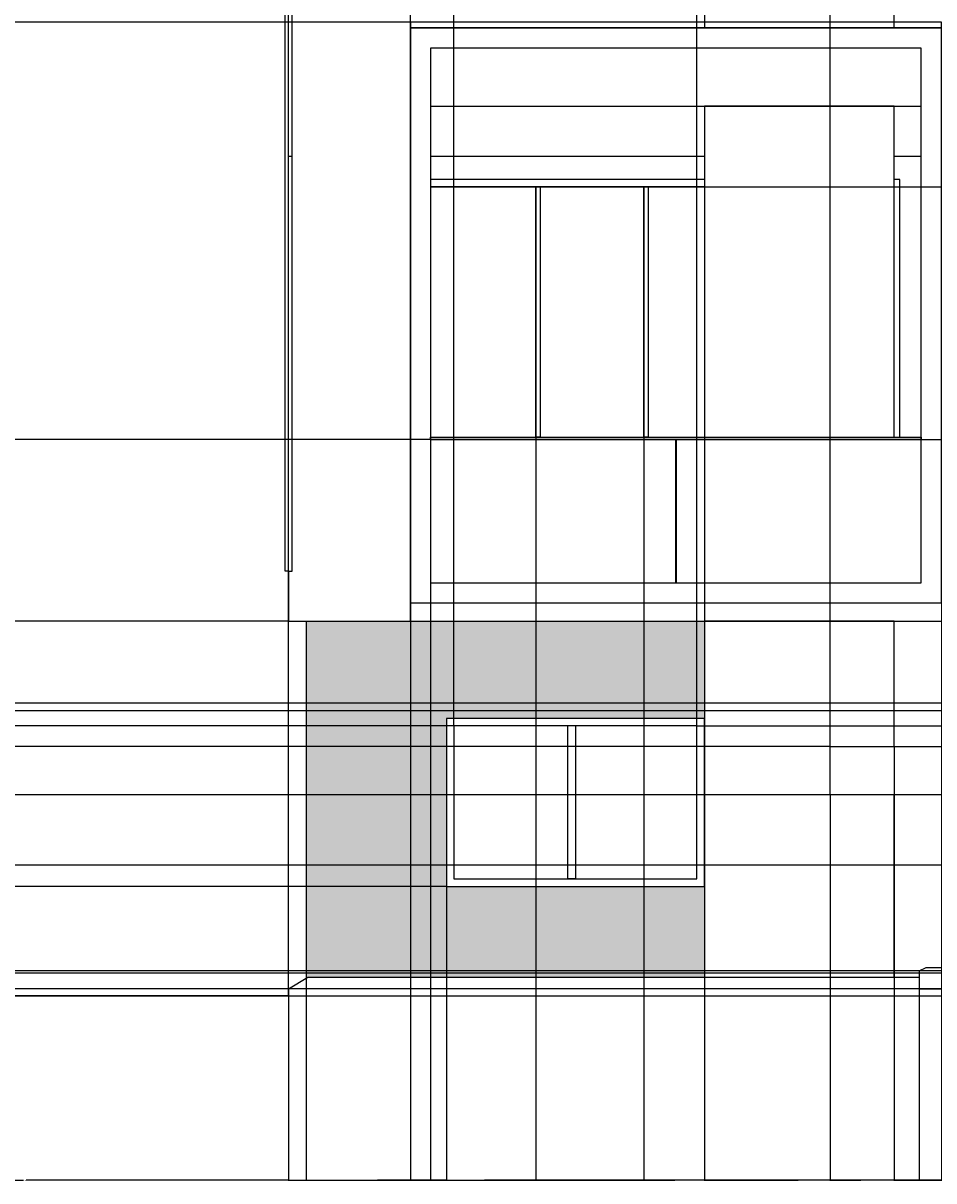
# Model space of a CAD drawing. Units: feet. Extents: x 2193 to 3502, y 890 to 1601.
# Tile 9 of 17: x 2848 to 3145, y 890 to 1268. Entities that reach past the tile are written whole.
import ezdxf

# ---------------------------------------------------------------- set-up
doc = ezdxf.new("R2010")
doc.units = ezdxf.units.FT
for name, color, linetype, lineweight in [('A-ANNO-DIMS', 2, 'Continuous', 18), ('A-ELEV', 7, 'Continuous', 25), ('A-ELEV-PATT', 8, 'Continuous', 13)]:
    doc.layers.add(name, color=color, linetype=linetype, lineweight=lineweight)
doc.styles.get("Standard").update_dxf_attribs({"font": 'arial.ttf'})
doc.dimstyles.get("Standard").update_dxf_attribs({"dimtxt": 0.18, "dimasz": 0.18, "dimexe": 0.18, "dimexo": 0.0625, "dimgap": 0.09, "dimtad": 0, "dimtih": 1, "dimtoh": 1, "dimdec": 0, "dimzin": 0, "dimdsep": 46, "dimlunit": 3, "dimtxsty": 'Standard', "dimcen": 0.09, "dimadec": 0, "dimazin": 0, "dimtfac": 1, "dimtdec": 0, "dimtofl": 0, "dimtmove": 0, "dimatfit": 3, "dimfxl": 1, "dimtolj": 1, "dimtzin": 0, "dimarcsym": 0})

# ---------------------------------------------------------------- blocks, each defined once
blk = doc.blocks.new('*D13')
at = {"layer": 'A-ANNO-DIMS', "color": 0, "lineweight": -2, "transparency": 16777216}
for p, q in [((2934.37, 950.89), (2934.37, 1601.47)), ((2934.55, 1601.29), (3186.64, 1601.29)), ((3439.51, 1601.29), (3187.43, 1601.29)), ((3439.69, 1541.11), (3439.69, 1601.47))]:
    blk.add_line(p, q, dxfattribs=at)
at = {"layer": 'A-ANNO-DIMS', "color": 0, "transparency": 16777216}
for points in [[(2934.55, 1601.32), (2934.55, 1601.26), (2934.37, 1601.29)], [(3439.51, 1601.32), (3439.51, 1601.26), (3439.69, 1601.29)]]:
    blk.add_solid(points, dxfattribs=at)
at = {"layer": 'Defpoints', "color": 0, "transparency": 16777216}
for p in [(3439.69, 1601.29), (3439.69, 1541.04), (2934.37, 950.82)]:
    blk.add_point(p, dxfattribs=at)
at = {"layer": 'A-ANNO-DIMS', "color": 0, "transparency": 16777216, "insert": (3187.03, 1601.29), "char_height": 0.18, "attachment_point": 5}
blk.add_mtext('\\A1;505.3', dxfattribs=at)
blk = doc.blocks.new('*D14')
at = {"layer": 'A-ANNO-DIMS', "color": 0, "lineweight": -2, "transparency": 16777216}
for p, q in [((3070.11, 956.87), (3070.11, 890.39)), ((2934.37, 950.76), (2934.37, 890.39)), ((2934.55, 890.57), (3001.79, 890.57)), ((3069.93, 890.57), (3002.7, 890.57))]:
    blk.add_line(p, q, dxfattribs=at)
at = {"layer": 'A-ANNO-DIMS', "color": 0, "transparency": 16777216}
for points in [[(2934.55, 890.6), (2934.55, 890.54), (2934.37, 890.57)], [(3069.93, 890.6), (3069.93, 890.54), (3070.11, 890.57)]]:
    blk.add_solid(points, dxfattribs=at)
at = {"layer": 'Defpoints', "color": 0, "transparency": 16777216}
for p in [(3070.11, 956.94), (2934.37, 950.82), (3070.11, 890.57)]:
    blk.add_point(p, dxfattribs=at)
at = {"layer": 'A-ANNO-DIMS', "color": 0, "transparency": 16777216, "insert": (3002.24, 890.57), "char_height": 0.18, "attachment_point": 5}
blk.add_mtext('\\A1;135.74', dxfattribs=at)
blk = doc.blocks.new('*D15')
at = {"layer": 'A-ANNO-DIMS', "color": 0, "lineweight": -2, "transparency": 16777216}
for p, q in [((3070.11, 956.87), (3070.11, 890.39)), ((3132, 956.87), (3132, 890.39)), ((3070.29, 890.57), (3100.66, 890.57)), ((3131.82, 890.57), (3101.45, 890.57))]:
    blk.add_line(p, q, dxfattribs=at)
at = {"layer": 'A-ANNO-DIMS', "color": 0, "transparency": 16777216}
for points in [[(3070.29, 890.6), (3070.29, 890.54), (3070.11, 890.57)], [(3131.82, 890.6), (3131.82, 890.54), (3132, 890.57)]]:
    blk.add_solid(points, dxfattribs=at)
at = {"layer": 'Defpoints', "color": 0, "transparency": 16777216}
for p in [(3070.11, 956.94), (3132, 956.94), (3132, 890.57)]:
    blk.add_point(p, dxfattribs=at)
at = {"layer": 'A-ANNO-DIMS', "color": 0, "transparency": 16777216, "insert": (3101.05, 890.57), "char_height": 0.18, "attachment_point": 5}
blk.add_mtext('\\A1;61.89', dxfattribs=at)
blk = doc.blocks.new('*D16')
at = {"layer": 'A-ANNO-DIMS', "color": 0, "lineweight": -2, "transparency": 16777216}
for p, q in [((3132, 956.87), (3132, 890.39)), ((3305.41, 950.76), (3305.41, 890.39)), ((3132.18, 890.57), (3218.32, 890.57)), ((3305.23, 890.57), (3219.09, 890.57))]:
    blk.add_line(p, q, dxfattribs=at)
at = {"layer": 'A-ANNO-DIMS', "color": 0, "transparency": 16777216}
for points in [[(3132.18, 890.6), (3132.18, 890.54), (3132, 890.57)], [(3305.23, 890.6), (3305.23, 890.54), (3305.41, 890.57)]]:
    blk.add_solid(points, dxfattribs=at)
at = {"layer": 'Defpoints', "color": 0, "transparency": 16777216}
for p in [(3132, 956.94), (3305.41, 950.82), (3305.41, 890.57)]:
    blk.add_point(p, dxfattribs=at)
at = {"layer": 'A-ANNO-DIMS', "color": 0, "transparency": 16777216, "insert": (3218.71, 890.57), "char_height": 0.18, "attachment_point": 5}
blk.add_mtext('\\A1;173.4', dxfattribs=at)
blk = doc.blocks.new('*D19')
at = {"layer": 'A-ANNO-DIMS', "color": 0, "lineweight": -2, "transparency": 16777216}
for p, q in [((2934.31, 1073.03), (2193.56, 1073.03)), ((2193.74, 1072.85), (2193.74, 1012.11)), ((2193.74, 951), (2193.74, 1011.75)), ((2934.31, 950.82), (2193.56, 950.82))]:
    blk.add_line(p, q, dxfattribs=at)
at = {"layer": 'A-ANNO-DIMS', "color": 0, "transparency": 16777216}
for points in [[(2193.71, 1072.85), (2193.77, 1072.85), (2193.74, 1073.03)], [(2193.71, 951), (2193.77, 951), (2193.74, 950.82)]]:
    blk.add_solid(points, dxfattribs=at)
at = {"layer": 'Defpoints', "color": 0, "transparency": 16777216}
for p in [(2193.74, 1073.03), (2934.37, 1073.03), (2934.37, 950.82)]:
    blk.add_point(p, dxfattribs=at)
at = {"layer": 'A-ANNO-DIMS', "color": 0, "transparency": 16777216, "insert": (2193.74, 1011.93), "char_height": 0.18, "attachment_point": 5}
blk.add_mtext('\\A1;122.2', dxfattribs=at)
blk = doc.blocks.new('*D20')
at = {"layer": 'A-ANNO-DIMS', "color": 0, "lineweight": -2, "transparency": 16777216}
for p, q in [((2933.15, 1408.48), (2193.56, 1408.48)), ((2193.74, 1408.3), (2193.74, 1240.94)), ((2193.74, 1073.21), (2193.74, 1240.57)), ((2934.31, 1073.03), (2193.56, 1073.03))]:
    blk.add_line(p, q, dxfattribs=at)
at = {"layer": 'A-ANNO-DIMS', "color": 0, "transparency": 16777216}
for points in [[(2193.71, 1408.3), (2193.77, 1408.3), (2193.74, 1408.48)], [(2193.71, 1073.21), (2193.77, 1073.21), (2193.74, 1073.03)]]:
    blk.add_solid(points, dxfattribs=at)
at = {"layer": 'Defpoints', "color": 0, "transparency": 16777216}
for p in [(2193.74, 1408.48), (2933.21, 1408.48), (2934.37, 1073.03)]:
    blk.add_point(p, dxfattribs=at)
at = {"layer": 'A-ANNO-DIMS', "color": 0, "transparency": 16777216, "insert": (2193.74, 1240.76), "char_height": 0.18, "attachment_point": 5}
blk.add_mtext('\\A1;335.45', dxfattribs=at)
blk = doc.blocks.new('*D22')
at = {"layer": 'A-ANNO-DIMS', "color": 0, "lineweight": -2, "transparency": 16777216}
for p, q in [((2988.31, 1038.93), (2988.31, 1601.47)), ((2988.49, 1601.29), (3027.59, 1601.29)), ((3067.48, 1601.29), (3028.38, 1601.29)), ((3067.66, 1038.93), (3067.66, 1601.47))]:
    blk.add_line(p, q, dxfattribs=at)
at = {"layer": 'A-ANNO-DIMS', "color": 0, "transparency": 16777216}
for points in [[(2988.49, 1601.32), (2988.49, 1601.26), (2988.31, 1601.29)], [(3067.48, 1601.32), (3067.48, 1601.26), (3067.66, 1601.29)]]:
    blk.add_solid(points, dxfattribs=at)
at = {"layer": 'Defpoints', "color": 0, "transparency": 16777216}
for p in [(3067.66, 1601.29), (2988.31, 1038.87), (3067.66, 1038.87)]:
    blk.add_point(p, dxfattribs=at)
at = {"layer": 'A-ANNO-DIMS', "color": 0, "transparency": 16777216, "insert": (3027.98, 1601.29), "char_height": 0.18, "attachment_point": 5}
blk.add_mtext('\\A1;79.36', dxfattribs=at)
blk = doc.blocks.new('*D23')
at = {"layer": 'A-ANNO-DIMS', "color": 0, "lineweight": -2, "transparency": 16777216}
for p, q in [((2988.24, 1038.87), (2193.56, 1038.87)), ((2193.74, 1038.69), (2193.74, 1012.87)), ((2193.74, 986.69), (2193.74, 1012.51)), ((2985.8, 986.51), (2193.56, 986.51))]:
    blk.add_line(p, q, dxfattribs=at)
at = {"layer": 'A-ANNO-DIMS', "color": 0, "transparency": 16777216}
for points in [[(2193.71, 1038.69), (2193.77, 1038.69), (2193.74, 1038.87)], [(2193.71, 986.69), (2193.77, 986.69), (2193.74, 986.51)]]:
    blk.add_solid(points, dxfattribs=at)
at = {"layer": 'Defpoints', "color": 0, "transparency": 16777216}
for p in [(2193.74, 1038.87), (2988.31, 1038.87), (2985.86, 986.51)]:
    blk.add_point(p, dxfattribs=at)
at = {"layer": 'A-ANNO-DIMS', "color": 0, "transparency": 16777216, "insert": (2193.74, 1012.69), "char_height": 0.18, "attachment_point": 5}
blk.add_mtext('\\A1;52.35', dxfattribs=at)
blk = doc.blocks.new('*D24')
at = {"layer": 'A-ANNO-DIMS', "color": 0, "lineweight": -2, "transparency": 16777216}
for p, q in [((2985.86, 986.45), (2985.86, 890.39)), ((2940.08, 956.47), (2940.08, 890.39)), ((2940.26, 890.57), (2962.57, 890.57)), ((2985.68, 890.57), (2963.37, 890.57))]:
    blk.add_line(p, q, dxfattribs=at)
at = {"layer": 'A-ANNO-DIMS', "color": 0, "transparency": 16777216}
for points in [[(2940.26, 890.6), (2940.26, 890.54), (2940.08, 890.57)], [(2985.68, 890.6), (2985.68, 890.54), (2985.86, 890.57)]]:
    blk.add_solid(points, dxfattribs=at)
at = {"layer": 'Defpoints', "color": 0, "transparency": 16777216}
for p in [(2985.86, 986.51), (2940.08, 956.53), (2985.86, 890.57)]:
    blk.add_point(p, dxfattribs=at)
at = {"layer": 'A-ANNO-DIMS', "color": 0, "transparency": 16777216, "insert": (2962.97, 890.57), "char_height": 0.18, "attachment_point": 5}
blk.add_mtext('\\A1;45.78', dxfattribs=at)
blk = doc.blocks.new('*D25')
at = {"layer": 'A-ANNO-DIMS', "color": 0, "lineweight": -2, "transparency": 16777216}
for p, q in [((3070.17, 1073.03), (3501.85, 1073.03)), ((3501.67, 1072.85), (3501.67, 1056.13)), ((3501.67, 1039.05), (3501.67, 1055.77)), ((3067.73, 1038.87), (3501.85, 1038.87))]:
    blk.add_line(p, q, dxfattribs=at)
at = {"layer": 'A-ANNO-DIMS', "color": 0, "transparency": 16777216}
for points in [[(3501.64, 1072.85), (3501.7, 1072.85), (3501.67, 1073.03)], [(3501.64, 1039.05), (3501.7, 1039.05), (3501.67, 1038.87)]]:
    blk.add_solid(points, dxfattribs=at)
at = {"layer": 'Defpoints', "color": 0, "transparency": 16777216}
for p in [(3070.11, 1073.03), (3501.67, 1073.03), (3067.66, 1038.87)]:
    blk.add_point(p, dxfattribs=at)
at = {"layer": 'A-ANNO-DIMS', "color": 0, "transparency": 16777216, "insert": (3501.67, 1055.95), "char_height": 0.18, "attachment_point": 5}
blk.add_mtext('\\A1;34.165', dxfattribs=at)
blk = doc.blocks.new('*D31')
at = {"layer": 'A-ANNO-DIMS', "color": 0, "lineweight": -2, "transparency": 16777216}
for p, q in [((2760.54, 1541.04), (3501.85, 1541.04)), ((3501.67, 1540.86), (3501.67, 1246.12)), ((3501.67, 951), (3501.67, 1245.75)), ((2762.27, 950.82), (3501.85, 950.82))]:
    blk.add_line(p, q, dxfattribs=at)
at = {"layer": 'A-ANNO-DIMS', "color": 0, "transparency": 16777216}
for points in [[(3501.64, 1540.86), (3501.7, 1540.86), (3501.67, 1541.04)], [(3501.64, 951), (3501.7, 951), (3501.67, 950.82)]]:
    blk.add_solid(points, dxfattribs=at)
at = {"layer": 'Defpoints', "color": 0, "transparency": 16777216}
for p in [(2760.47, 1541.04), (3501.67, 1541.04), (2762.2, 950.82)]:
    blk.add_point(p, dxfattribs=at)
at = {"layer": 'A-ANNO-DIMS', "color": 0, "transparency": 16777216, "insert": (3501.67, 1245.93), "char_height": 0.18, "attachment_point": 5}
blk.add_mtext('\\A1;590.2', dxfattribs=at)
blk = doc.blocks.new('*D35')
at = {"layer": 'A-ANNO-DIMS', "color": 0, "lineweight": -2, "transparency": 16777216}
for p, q in [((2980.65, 1132.39), (2193.56, 1132.39)), ((2193.74, 1132.21), (2193.74, 1102.89)), ((2193.74, 1073.21), (2193.74, 1102.53)), ((2934.31, 1073.03), (2193.56, 1073.03))]:
    blk.add_line(p, q, dxfattribs=at)
at = {"layer": 'A-ANNO-DIMS', "color": 0, "transparency": 16777216}
for points in [[(2193.71, 1132.21), (2193.77, 1132.21), (2193.74, 1132.39)], [(2193.71, 1073.21), (2193.77, 1073.21), (2193.74, 1073.03)]]:
    blk.add_solid(points, dxfattribs=at)
at = {"layer": 'Defpoints', "color": 0, "transparency": 16777216}
for p in [(2193.74, 1132.39), (2980.72, 1132.39), (2934.37, 1073.03)]:
    blk.add_point(p, dxfattribs=at)
at = {"layer": 'A-ANNO-DIMS', "color": 0, "transparency": 16777216, "insert": (2193.74, 1102.71), "char_height": 0.18, "attachment_point": 5}
blk.add_mtext('\\A1;59.36', dxfattribs=at)
blk = doc.blocks.new('*D36')
at = {"layer": 'A-ANNO-DIMS', "color": 0, "lineweight": -2, "transparency": 16777216}
for p, q in [((2974.05, 1268.66), (2193.56, 1268.66)), ((2193.74, 1268.48), (2193.74, 1200.71)), ((2193.74, 1132.57), (2193.74, 1200.34)), ((2980.65, 1132.39), (2193.56, 1132.39))]:
    blk.add_line(p, q, dxfattribs=at)
at = {"layer": 'A-ANNO-DIMS', "color": 0, "transparency": 16777216}
for points in [[(2193.71, 1268.48), (2193.77, 1268.48), (2193.74, 1268.66)], [(2193.71, 1132.57), (2193.77, 1132.57), (2193.74, 1132.39)]]:
    blk.add_solid(points, dxfattribs=at)
at = {"layer": 'Defpoints', "color": 0, "transparency": 16777216}
for p in [(2193.74, 1268.66), (2974.12, 1268.66), (2980.72, 1132.39)]:
    blk.add_point(p, dxfattribs=at)
at = {"layer": 'A-ANNO-DIMS', "color": 0, "transparency": 16777216, "insert": (2193.74, 1200.53), "char_height": 0.18, "attachment_point": 5}
blk.add_mtext('\\A1;136.27', dxfattribs=at)
blk = doc.blocks.new('*D61')
at = {"layer": 'A-ANNO-DIMS', "color": 0, "lineweight": -2, "transparency": 16777216}
for p, q in [((2974.12, 1078.97), (2974.12, 890.39)), ((3147.5, 1078.97), (3147.5, 890.39)), ((2974.3, 890.57), (3060.42, 890.57)), ((3147.32, 890.57), (3061.19, 890.57))]:
    blk.add_line(p, q, dxfattribs=at)
at = {"layer": 'A-ANNO-DIMS', "color": 0, "transparency": 16777216}
for points in [[(2974.3, 890.6), (2974.3, 890.54), (2974.12, 890.57)], [(3147.32, 890.6), (3147.32, 890.54), (3147.5, 890.57)]]:
    blk.add_solid(points, dxfattribs=at)
at = {"layer": 'Defpoints', "color": 0, "transparency": 16777216}
for p in [(2974.12, 1079.03), (3147.5, 1079.03), (3147.5, 890.57)]:
    blk.add_point(p, dxfattribs=at)
at = {"layer": 'A-ANNO-DIMS', "color": 0, "transparency": 16777216, "insert": (3060.81, 890.57), "char_height": 0.18, "attachment_point": 5}
blk.add_mtext('\\A1;173.4', dxfattribs=at)
blk = doc.blocks.new('*D62')
at = {"layer": 'A-ANNO-DIMS', "color": 0, "lineweight": -2, "transparency": 16777216}
for p, q in [((2974.18, 1266.71), (3501.85, 1266.71)), ((3501.67, 1266.53), (3501.67, 1173.05)), ((3501.67, 1079.21), (3501.67, 1172.69)), ((2974.18, 1079.03), (3501.85, 1079.03))]:
    blk.add_line(p, q, dxfattribs=at)
at = {"layer": 'A-ANNO-DIMS', "color": 0, "transparency": 16777216}
for points in [[(3501.64, 1266.53), (3501.7, 1266.53), (3501.67, 1266.71)], [(3501.64, 1079.21), (3501.7, 1079.21), (3501.67, 1079.03)]]:
    blk.add_solid(points, dxfattribs=at)
at = {"layer": 'Defpoints', "color": 0, "transparency": 16777216}
for p in [(2974.12, 1266.71), (3501.67, 1266.71), (2974.12, 1079.03)]:
    blk.add_point(p, dxfattribs=at)
at = {"layer": 'A-ANNO-DIMS', "color": 0, "transparency": 16777216, "insert": (3501.67, 1172.87), "char_height": 0.18, "attachment_point": 5}
blk.add_mtext('\\A1;187.68', dxfattribs=at)
blk = doc.blocks.new('*D63')
at = {"layer": 'A-ANNO-DIMS', "color": 0, "lineweight": -2, "transparency": 16777216}
for p, q in [((2980.72, 1085.57), (2980.72, 890.39)), ((2974.12, 1078.97), (2974.12, 890.39)), ((2974.3, 890.57), (2977.02, 890.57)), ((2980.54, 890.57), (2977.81, 890.57))]:
    blk.add_line(p, q, dxfattribs=at)
at = {"layer": 'A-ANNO-DIMS', "color": 0, "transparency": 16777216}
for points in [[(2974.3, 890.6), (2974.3, 890.54), (2974.12, 890.57)], [(2980.54, 890.6), (2980.54, 890.54), (2980.72, 890.57)]]:
    blk.add_solid(points, dxfattribs=at)
at = {"layer": 'Defpoints', "color": 0, "transparency": 16777216}
for p in [(2980.72, 1085.63), (2974.12, 1079.03), (2980.72, 890.57)]:
    blk.add_point(p, dxfattribs=at)
at = {"layer": 'A-ANNO-DIMS', "color": 0, "transparency": 16777216, "insert": (2977.42, 890.57), "char_height": 0.18, "attachment_point": 5}
blk.add_mtext('\\A1;6.599', dxfattribs=at)
blk = doc.blocks.new('*D64')
at = {"layer": 'A-ANNO-DIMS', "color": 0, "lineweight": -2, "transparency": 16777216}
for p, q in [((2980.72, 1214.77), (2980.72, 890.39)), ((3015.08, 1214.77), (3015.08, 890.39)), ((2980.9, 890.57), (2997.43, 890.57)), ((3014.9, 890.57), (2998.36, 890.57))]:
    blk.add_line(p, q, dxfattribs=at)
at = {"layer": 'A-ANNO-DIMS', "color": 0, "transparency": 16777216}
for points in [[(2980.9, 890.6), (2980.9, 890.54), (2980.72, 890.57)], [(3014.9, 890.6), (3014.9, 890.54), (3015.08, 890.57)]]:
    blk.add_solid(points, dxfattribs=at)
at = {"layer": 'Defpoints', "color": 0, "transparency": 16777216}
for p in [(2980.72, 1214.84), (3015.08, 1214.84), (3015.08, 890.57)]:
    blk.add_point(p, dxfattribs=at)
at = {"layer": 'A-ANNO-DIMS', "color": 0, "transparency": 16777216, "insert": (2997.9, 890.57), "char_height": 0.18, "attachment_point": 5}
blk.add_mtext('\\A1;34.365', dxfattribs=at)
blk = doc.blocks.new('*D65')
at = {"layer": 'A-ANNO-DIMS', "color": 0, "lineweight": -2, "transparency": 16777216}
for p, q in [((3015.08, 1214.77), (3015.08, 890.39)), ((3050.34, 1214.77), (3050.34, 890.39)), ((3015.26, 890.57), (3032.32, 890.57)), ((3050.16, 890.57), (3033.1, 890.57))]:
    blk.add_line(p, q, dxfattribs=at)
at = {"layer": 'A-ANNO-DIMS', "color": 0, "transparency": 16777216}
for points in [[(3015.26, 890.6), (3015.26, 890.54), (3015.08, 890.57)], [(3050.16, 890.6), (3050.16, 890.54), (3050.34, 890.57)]]:
    blk.add_solid(points, dxfattribs=at)
at = {"layer": 'Defpoints', "color": 0, "transparency": 16777216}
for p in [(3015.08, 1214.84), (3050.34, 1214.84), (3050.34, 890.57)]:
    blk.add_point(p, dxfattribs=at)
at = {"layer": 'A-ANNO-DIMS', "color": 0, "transparency": 16777216, "insert": (3032.71, 890.57), "char_height": 0.18, "attachment_point": 5}
blk.add_mtext('\\A1;35.26', dxfattribs=at)
blk = doc.blocks.new('*D66')
at = {"layer": 'A-ANNO-DIMS', "color": 0, "lineweight": -2, "transparency": 16777216}
for p, q in [((3050.34, 1214.77), (3050.34, 890.39)), ((3070.11, 1214.77), (3070.11, 890.39)), ((3050.52, 890.57), (3059.84, 890.57)), ((3069.93, 890.57), (3060.61, 890.57))]:
    blk.add_line(p, q, dxfattribs=at)
at = {"layer": 'A-ANNO-DIMS', "color": 0, "transparency": 16777216}
for points in [[(3050.52, 890.6), (3050.52, 890.54), (3050.34, 890.57)], [(3069.93, 890.6), (3069.93, 890.54), (3070.11, 890.57)]]:
    blk.add_solid(points, dxfattribs=at)
at = {"layer": 'Defpoints', "color": 0, "transparency": 16777216}
for p in [(3050.34, 1214.84), (3070.11, 1214.84), (3070.11, 890.57)]:
    blk.add_point(p, dxfattribs=at)
at = {"layer": 'A-ANNO-DIMS', "color": 0, "transparency": 16777216, "insert": (3060.23, 890.57), "char_height": 0.18, "attachment_point": 5}
blk.add_mtext('\\A1;19.77', dxfattribs=at)
blk = doc.blocks.new('*D67')
at = {"layer": 'A-ANNO-DIMS', "color": 0, "lineweight": -2, "transparency": 16777216}
for p, q in [((2980.78, 1214.84), (3501.85, 1214.84)), ((3501.67, 1214.66), (3501.67, 1173.8)), ((3501.67, 1132.57), (3501.67, 1173.43)), ((2980.78, 1132.39), (3501.85, 1132.39))]:
    blk.add_line(p, q, dxfattribs=at)
at = {"layer": 'A-ANNO-DIMS', "color": 0, "transparency": 16777216}
for points in [[(3501.64, 1214.66), (3501.7, 1214.66), (3501.67, 1214.84)], [(3501.64, 1132.57), (3501.7, 1132.57), (3501.67, 1132.39)]]:
    blk.add_solid(points, dxfattribs=at)
at = {"layer": 'Defpoints', "color": 0, "transparency": 16777216}
for p in [(2980.72, 1214.84), (3501.67, 1214.84), (2980.72, 1132.39)]:
    blk.add_point(p, dxfattribs=at)
at = {"layer": 'A-ANNO-DIMS', "color": 0, "transparency": 16777216, "insert": (3501.67, 1173.62), "char_height": 0.18, "attachment_point": 5}
blk.add_mtext('\\A1;82.44', dxfattribs=at)
blk = doc.blocks.new('*D97')
at = {"layer": 'A-ANNO-DIMS', "color": 0, "lineweight": -2, "transparency": 16777216}
for p, q in [((3111.13, 1032.26), (3111.13, 1601.47)), ((3111.31, 1601.29), (3207.6, 1601.29)), ((3304.79, 1601.29), (3208.51, 1601.29)), ((3304.97, 1032.26), (3304.97, 1601.47))]:
    blk.add_line(p, q, dxfattribs=at)
at = {"layer": 'A-ANNO-DIMS', "color": 0, "transparency": 16777216}
for points in [[(3111.31, 1601.32), (3111.31, 1601.26), (3111.13, 1601.29)], [(3304.79, 1601.32), (3304.79, 1601.26), (3304.97, 1601.29)]]:
    blk.add_solid(points, dxfattribs=at)
at = {"layer": 'Defpoints', "color": 0, "transparency": 16777216}
for p in [(3304.97, 1601.29), (3111.13, 1032.19), (3304.97, 1032.19)]:
    blk.add_point(p, dxfattribs=at)
at = {"layer": 'A-ANNO-DIMS', "color": 0, "transparency": 16777216, "insert": (3208.05, 1601.29), "char_height": 0.18, "attachment_point": 5}
blk.add_mtext('\\A1;193.84', dxfattribs=at)
blk = doc.blocks.new('*D98')
at = {"layer": 'A-ANNO-DIMS', "color": 0, "lineweight": -2, "transparency": 16777216}
for p, q in [((3111.07, 1032.19), (2193.56, 1032.19)), ((2193.74, 1032.01), (2193.74, 1024.48)), ((2193.74, 1016.58), (2193.74, 1024.11)), ((3111.07, 1016.4), (2193.56, 1016.4))]:
    blk.add_line(p, q, dxfattribs=at)
at = {"layer": 'A-ANNO-DIMS', "color": 0, "transparency": 16777216}
for points in [[(2193.71, 1032.01), (2193.77, 1032.01), (2193.74, 1032.19)], [(2193.71, 1016.58), (2193.77, 1016.58), (2193.74, 1016.4)]]:
    blk.add_solid(points, dxfattribs=at)
at = {"layer": 'Defpoints', "color": 0, "transparency": 16777216}
for p in [(2193.74, 1032.19), (3111.13, 1032.19), (3111.13, 1016.4)]:
    blk.add_point(p, dxfattribs=at)
at = {"layer": 'A-ANNO-DIMS', "color": 0, "transparency": 16777216, "insert": (2193.74, 1024.3), "char_height": 0.18, "attachment_point": 5}
blk.add_mtext('\\A1;15.793', dxfattribs=at)
blk = doc.blocks.new('*D99')
at = {"layer": 'A-ANNO-DIMS', "color": 0, "lineweight": -2, "transparency": 16777216}
for p, q in [((3111.13, 1016.34), (3111.13, 890.39)), ((3132, 1016.34), (3132, 890.39)), ((3111.31, 890.57), (3121.17, 890.57)), ((3131.82, 890.57), (3121.96, 890.57))]:
    blk.add_line(p, q, dxfattribs=at)
at = {"layer": 'A-ANNO-DIMS', "color": 0, "transparency": 16777216}
for points in [[(3111.31, 890.6), (3111.31, 890.54), (3111.13, 890.57)], [(3131.82, 890.6), (3131.82, 890.54), (3132, 890.57)]]:
    blk.add_solid(points, dxfattribs=at)
at = {"layer": 'Defpoints', "color": 0, "transparency": 16777216}
for p in [(3111.13, 1016.4), (3132, 1016.4), (3132, 890.57)]:
    blk.add_point(p, dxfattribs=at)
at = {"layer": 'A-ANNO-DIMS', "color": 0, "transparency": 16777216, "insert": (3121.56, 890.57), "char_height": 0.18, "attachment_point": 5}
blk.add_mtext('\\A1;20.87', dxfattribs=at)
blk = doc.blocks.new('*D102')
at = {"layer": 'A-ANNO-DIMS', "color": 0, "lineweight": -2, "transparency": 16777216}
for p, q in [((3132, 1032.13), (3132, 890.39)), ((3168.83, 1032.13), (3168.83, 890.39)), ((3132.18, 890.57), (3149.95, 890.57)), ((3168.65, 890.57), (3150.88, 890.57))]:
    blk.add_line(p, q, dxfattribs=at)
at = {"layer": 'A-ANNO-DIMS', "color": 0, "transparency": 16777216}
for points in [[(3132.18, 890.6), (3132.18, 890.54), (3132, 890.57)], [(3168.65, 890.6), (3168.65, 890.54), (3168.83, 890.57)]]:
    blk.add_solid(points, dxfattribs=at)
at = {"layer": 'Defpoints', "color": 0, "transparency": 16777216}
for p in [(3132, 1032.19), (3168.83, 1032.19), (3168.83, 890.57)]:
    blk.add_point(p, dxfattribs=at)
at = {"layer": 'A-ANNO-DIMS', "color": 0, "transparency": 16777216, "insert": (3150.42, 890.57), "char_height": 0.18, "attachment_point": 5}
blk.add_mtext('\\A1;36.835', dxfattribs=at)
blk = doc.blocks.new('*D107')
at = {"layer": 'A-ANNO-DIMS', "color": 0, "lineweight": -2, "transparency": 16777216}
for p, q in [((3140.22, 958.89), (3140.22, 890.39)), ((3159.3, 958.89), (3159.3, 890.39)), ((3140.4, 890.57), (3149.3, 890.57)), ((3159.12, 890.57), (3150.22, 890.57))]:
    blk.add_line(p, q, dxfattribs=at)
at = {"layer": 'A-ANNO-DIMS', "color": 0, "transparency": 16777216}
for points in [[(3140.4, 890.6), (3140.4, 890.54), (3140.22, 890.57)], [(3159.12, 890.6), (3159.12, 890.54), (3159.3, 890.57)]]:
    blk.add_solid(points, dxfattribs=at)
at = {"layer": 'Defpoints', "color": 0, "transparency": 16777216}
for p in [(3140.22, 958.96), (3159.3, 958.96), (3159.3, 890.57)]:
    blk.add_point(p, dxfattribs=at)
at = {"layer": 'A-ANNO-DIMS', "color": 0, "transparency": 16777216, "insert": (3149.76, 890.57), "char_height": 0.18, "attachment_point": 5}
blk.add_mtext('\\A1;19.075', dxfattribs=at)
blk = doc.blocks.new('*D116')
at = {"layer": 'A-ANNO-DIMS', "color": 0, "lineweight": -2, "transparency": 16777216}
for p, q in [((3140.16, 958.96), (2193.56, 958.96)), ((2193.74, 958.78), (2193.74, 956.18)), ((3140.16, 953.03), (2193.56, 953.03)), ((2193.74, 953.21), (2193.74, 955.81))]:
    blk.add_line(p, q, dxfattribs=at)
at = {"layer": 'A-ANNO-DIMS', "color": 0, "transparency": 16777216}
for points in [[(2193.71, 958.78), (2193.77, 958.78), (2193.74, 958.96)], [(2193.71, 953.21), (2193.77, 953.21), (2193.74, 953.03)]]:
    blk.add_solid(points, dxfattribs=at)
at = {"layer": 'Defpoints', "color": 0, "transparency": 16777216}
for p in [(2193.74, 958.96), (3140.22, 958.96), (3140.22, 953.03)]:
    blk.add_point(p, dxfattribs=at)
at = {"layer": 'A-ANNO-DIMS', "color": 0, "transparency": 16777216, "insert": (2193.74, 955.99), "char_height": 0.18, "attachment_point": 5}
blk.add_mtext('\\A1;5.924', dxfattribs=at)
blk = doc.blocks.new('*D124')
at = {"layer": 'A-ANNO-DIMS', "color": 0, "lineweight": -2, "transparency": 16777216}
for p, q in [((3304.91, 1046.36), (2193.56, 1046.36)), ((3304.91, 1043.78), (2193.56, 1043.78)), ((2193.74, 1046.18), (2193.74, 1045.26)), ((2193.74, 1043.96), (2193.74, 1044.89))]:
    blk.add_line(p, q, dxfattribs=at)
at = {"layer": 'A-ANNO-DIMS', "color": 0, "transparency": 16777216}
for points in [[(2193.71, 1046.18), (2193.77, 1046.18), (2193.74, 1046.36)], [(2193.71, 1043.96), (2193.77, 1043.96), (2193.74, 1043.78)]]:
    blk.add_solid(points, dxfattribs=at)
at = {"layer": 'Defpoints', "color": 0, "transparency": 16777216}
for p in [(2193.74, 1043.78), (3304.97, 1046.36), (3304.97, 1043.78)]:
    blk.add_point(p, dxfattribs=at)
at = {"layer": 'A-ANNO-DIMS', "color": 0, "transparency": 16777216, "insert": (2193.74, 1045.07), "char_height": 0.18, "attachment_point": 5}
blk.add_mtext('\\A1;2.583', dxfattribs=at)
blk = doc.blocks.new('*D126')
at = {"layer": 'A-ANNO-DIMS', "color": 0, "lineweight": -2, "transparency": 16777216}
for p, q in [((2762.2, 950.76), (2762.2, 890.39)), ((2934.37, 950.76), (2934.37, 890.39)), ((2762.38, 890.57), (2847.83, 890.57)), ((2934.19, 890.57), (2848.74, 890.57))]:
    blk.add_line(p, q, dxfattribs=at)
at = {"layer": 'A-ANNO-DIMS', "color": 0, "transparency": 16777216}
for points in [[(2762.38, 890.6), (2762.38, 890.54), (2762.2, 890.57)], [(2934.19, 890.6), (2934.19, 890.54), (2934.37, 890.57)]]:
    blk.add_solid(points, dxfattribs=at)
at = {"layer": 'Defpoints', "color": 0, "transparency": 16777216}
for p in [(2762.2, 950.82), (2934.37, 950.82), (2934.37, 890.57)]:
    blk.add_point(p, dxfattribs=at)
at = {"layer": 'A-ANNO-DIMS', "color": 0, "transparency": 16777216, "insert": (2848.29, 890.57), "char_height": 0.18, "attachment_point": 5}
blk.add_mtext('\\A1;172.17', dxfattribs=at)
blk = doc.blocks.new('*D130')
at = {"layer": 'A-ANNO-DIMS', "color": 0, "lineweight": -2, "transparency": 16777216}
for p, q in [((3304.91, 993.39), (2193.56, 993.39)), ((2193.74, 993.21), (2193.74, 975.95)), ((2193.74, 958.33), (2193.74, 975.59)), ((3304.91, 958.15), (2193.56, 958.15))]:
    blk.add_line(p, q, dxfattribs=at)
at = {"layer": 'A-ANNO-DIMS', "color": 0, "transparency": 16777216}
for points in [[(2193.71, 993.21), (2193.77, 993.21), (2193.74, 993.39)], [(2193.71, 958.33), (2193.77, 958.33), (2193.74, 958.15)]]:
    blk.add_solid(points, dxfattribs=at)
at = {"layer": 'Defpoints', "color": 0, "transparency": 16777216}
for p in [(2193.74, 993.39), (3304.97, 993.39), (3304.97, 958.15)]:
    blk.add_point(p, dxfattribs=at)
at = {"layer": 'A-ANNO-DIMS', "color": 0, "transparency": 16777216, "insert": (2193.74, 975.77), "char_height": 0.18, "attachment_point": 5}
blk.add_mtext('\\A1;35.24', dxfattribs=at)

msp = doc.modelspace()

# ---------------------------------------------------------------- hatches: boundary and pattern name
at = {"layer": 'A-ELEV-PATT'}
h = msp.add_hatch(color=256, dxfattribs=at)
h.dxf.hatch_style = 1
h.paths.add_polyline_path([(2622.9814, 1355.2199), (2452.7821, 1355.2199), (2452.7821, 1268.6599), (2468.2854, 1268.6599), (2468.2854, 1325.6699), (2579.767, 1325.6699), (2579.767, 1268.6599), (2622.9814, 1268.6599)])
h.paths.add_polyline_path([(2598.591, 1224.865), (2468.2854, 1224.865), (2468.2854, 1190.8659), (2579.767, 1190.8659), (2579.767, 1133.8558), (2598.591, 1133.8558)])
h.paths.add_polyline_path([(2390.8933, 1241.1967), (2301.4984, 1241.1967), (2301.4984, 1224.865), (2390.8933, 1224.865)])
h.paths.add_polyline_path([(3070.1101, 1073.031), (2940.0814, 1073.031), (2940.0814, 956.5285), (2940.6598, 956.8829), (3070.1101, 956.8829), (3070.1101, 986.5146), (2985.8599, 986.5146), (2985.8599, 1041.3109), (3070.1101, 1041.3109)])

# ---------------------------------------------------------------- linework, layer by layer
at = {"layer": 'A-ELEV'}
for p, q in [((2980.7151, 1241.1967), (3140.903, 1241.1967)), ((2934.3742, 1224.865), (2935.5399, 1224.865)), ((2980.7151, 1224.865), (3070.1101, 1224.865)), ((3131.9988, 1224.865), (3140.903, 1224.865)), ((2934.3742, 953.031), (2934.3742, 1089.3627)), ((2934.3742, 1089.3627), (2935.5399, 1089.3627)), ((2934.3742, 1073.031), (3439.6901, 1073.031)), ((3140.2223, 958.9555), (3142.4884, 960.0129)), ((3142.4884, 960.0129), (3159.2977, 960.0129)), ((2934.3742, 953.031), (2940.6598, 956.8829)), ((2940.6598, 956.8829), (3140.2223, 956.8829))]:
    msp.add_line(p, q, dxfattribs=at)
for points in [[(2934.3742, 1089.3627), (2933.2085, 1089.3627), (2933.2085, 1408.4814), (2934.3742, 1408.4814)], [(2934.3742, 1089.3627), (2935.5399, 1089.3627), (2935.5399, 1406.15)], [(2934.3742, 1089.3627), (2934.3742, 1073.031), (2974.116, 1073.031), (2974.116, 1367.5739)], [(3070.1101, 1367.5739), (3070.1101, 1266.7092), (3131.9988, 1266.7092), (3131.9988, 1355.2199)], [(3131.9988, 1133.1367), (3131.9988, 1241.1967), (3070.1101, 1241.1967), (3070.1101, 1133.1367)], [(3070.1101, 1217.2819), (2980.7151, 1217.2819), (2980.7151, 1133.1367)], [(3133.8383, 1133.1367), (3133.8383, 1217.2819), (3131.9988, 1217.2819)], [(3070.1101, 1214.8367), (2980.7151, 1214.8367)], [(2934.3742, 953.031), (2934.3742, 1073.031), (3070.1101, 1073.031), (3070.1101, 956.9371)], [(2934.3742, 953.031), (2934.3742, 1073.031), (2940.0814, 1073.031), (2940.0814, 956.5285)], [(3131.9988, 1032.1935), (3131.9988, 1073.031), (3070.1101, 1073.031), (3070.1101, 956.9371)], [(3027.985, 1038.8658), (3027.985, 988.9597), (3025.5399, 988.9597), (3025.5399, 1038.8658)], [(3111.1302, 1016.4), (3111.1302, 1032.1935), (3304.9731, 1032.1935), (3304.9731, 956.8829)], [(3279.6085, 953.031), (3279.6085, 1016.4), (3111.1302, 1016.4)], [(3131.9988, 956.9371), (3131.9988, 1016.4)]]:
    msp.add_lwpolyline(points, dxfattribs=at)
for points in [[(2974.116, 1266.7092), (3147.5022, 1266.7092), (3147.5022, 1268.6599), (2974.116, 1268.6599)], [(2974.116, 1079.031), (3147.5022, 1079.031), (3147.5022, 1266.7092), (2974.116, 1266.7092)], [(2980.7151, 1085.6301), (3140.903, 1085.6301), (3140.903, 1260.11), (2980.7151, 1260.11)], [(3015.08, 1214.8367), (3016.449, 1214.8367), (3016.449, 1133.1367), (3015.08, 1133.1367)], [(3050.3413, 1214.8367), (3051.7104, 1214.8367), (3051.7104, 1133.1367), (3050.3413, 1133.1367)], [(2980.7151, 1133.1367), (3140.903, 1133.1367), (3140.903, 1132.3937), (2980.7151, 1132.3937)], [(3060.6842, 1085.6301), (3060.9339, 1085.6301), (3060.9339, 1132.3937), (3060.6842, 1132.3937)], [(3070.1101, 1041.3109), (2985.8599, 1041.3109), (2985.8599, 986.5146), (3070.1101, 986.5146)], [(3067.665, 1038.8658), (2988.305, 1038.8658), (2988.305, 988.9597), (3067.665, 988.9597)], [(3140.2223, 953.031), (3266.9251, 953.031), (3266.9251, 958.9555), (3140.2223, 958.9555)], [(2934.3742, 950.8228), (3305.4139, 950.8228), (3305.4139, 953.031), (2934.3742, 953.031)]]:
    msp.add_lwpolyline(points, close=True, dxfattribs=at)

# ---------------------------------------------------------------- dimensions: what is measured, and where the dimension line sits
at = {"layer": 'A-ANNO-DIMS'}
for base, p1, p2, override, picture, middle in [((3439.6901, 1601.2941), (2934.3742, 950.8228), (3439.6901, 1541.0441), {"dimdec": 1, "dimlfac": 1, "dimrnd": 0, "dimzin": 0, "dimdsep": 46, "dimlunit": 2}, '*D13', (3187.0321, 1601.2941)), ((3067.665, 1601.2941), (2988.305, 1038.8658), (3067.665, 1038.8658), {"dimdec": 2, "dimlfac": 1, "dimrnd": 0, "dimzin": 0, "dimdsep": 46, "dimlunit": 2}, '*D22', (3027.985, 1601.2941)), ((3304.9731, 1601.2941), (3111.1302, 1032.1935), (3304.9731, 1032.1935), {"dimdec": 2, "dimlfac": 1, "dimrnd": 0, "dimzin": 0, "dimdsep": 46, "dimlunit": 2}, '*D97', (3208.0516, 1601.2941)), ((3015.08, 890.5728), (2980.7151, 1214.8367), (3015.08, 1214.8367), {"dimdec": 3, "dimlfac": 1, "dimrnd": 0, "dimzin": 0, "dimdsep": 46, "dimlunit": 2}, '*D64', (2997.8976, 890.5728)), ((3050.3413, 890.5728), (3015.08, 1214.8367), (3050.3413, 1214.8367), {"dimdec": 2, "dimlfac": 1, "dimrnd": 0, "dimzin": 0, "dimdsep": 46, "dimlunit": 2}, '*D65', (3032.7107, 890.5728)), ((3070.1101, 890.5728), (3050.3413, 1214.8367), (3070.1101, 1214.8367), {"dimdec": 2, "dimlfac": 1, "dimrnd": 0, "dimzin": 0, "dimdsep": 46, "dimlunit": 2}, '*D66', (3060.2257, 890.5728)), ((2980.7151, 890.5728), (2974.116, 1079.031), (2980.7151, 1085.6301), {"dimdec": 3, "dimlfac": 1, "dimrnd": 0, "dimzin": 0, "dimdsep": 46, "dimlunit": 2}, '*D63', (2977.4156, 890.5728)), ((3147.5022, 890.5728), (2974.116, 1079.031), (3147.5022, 1079.031), {"dimdec": 1, "dimlfac": 1, "dimrnd": 0, "dimzin": 0, "dimdsep": 46, "dimlunit": 2}, '*D61', (3060.8091, 890.5728)), ((3168.8336, 890.5728), (3131.9988, 1032.1935), (3168.8336, 1032.1935), {"dimdec": 3, "dimlfac": 1, "dimrnd": 0, "dimzin": 0, "dimdsep": 46, "dimlunit": 2}, '*D102', (3150.4162, 890.5728)), ((3131.9988, 890.5728), (3111.1302, 1016.4), (3131.9988, 1016.4), {"dimdec": 2, "dimlfac": 1, "dimrnd": 0, "dimzin": 0, "dimdsep": 46, "dimlunit": 2}, '*D99', (3121.5645, 890.5728)), ((2985.8599, 890.5728), (2940.0814, 956.5285), (2985.8599, 986.5146), {"dimdec": 2, "dimlfac": 1, "dimrnd": 0, "dimzin": 0, "dimdsep": 46, "dimlunit": 2}, '*D24', (2962.9707, 890.5728)), ((3070.1101, 890.5728), (2934.3742, 950.8228), (3070.1101, 956.9371), {"dimdec": 2, "dimlfac": 1, "dimrnd": 0, "dimzin": 0, "dimdsep": 46, "dimlunit": 2}, '*D14', (3002.2421, 890.5728)), ((3131.9988, 890.5728), (3070.1101, 956.9371), (3131.9988, 956.9371), {"dimdec": 2, "dimlfac": 1, "dimrnd": 0, "dimzin": 0, "dimdsep": 46, "dimlunit": 2}, '*D15', (3101.0545, 890.5728)), ((3305.4139, 890.5728), (3131.9988, 956.9371), (3305.4139, 950.8228), {"dimdec": 1, "dimlfac": 1, "dimrnd": 0, "dimzin": 0, "dimdsep": 46, "dimlunit": 2}, '*D16', (3218.7064, 890.5728)), ((3159.2977, 890.5728), (3140.2223, 958.9555), (3159.2977, 958.9555), {"dimdec": 3, "dimlfac": 1, "dimrnd": 0, "dimzin": 0, "dimdsep": 46, "dimlunit": 2}, '*D107', (3149.76, 890.5728)), ((2934.3742, 890.5728), (2762.2048, 950.8228), (2934.3742, 950.8228), {"dimdec": 2, "dimlfac": 1, "dimrnd": 0, "dimzin": 0, "dimdsep": 46, "dimlunit": 2}, '*D126', (2848.2895, 890.5728))]:
    dim = msp.add_linear_dim(base=base, p1=p1, p2=p2, dimstyle='Standard', override=override, dxfattribs=at)
    dim.commit()
    dim.dimension.update_dxf_attribs({"geometry": picture, "text_midpoint": middle})
for base, p1, p2, override, picture, middle in [((3501.6716, 1541.0441), (2762.2048, 950.8228), (2760.4733, 1541.0441), {"dimdec": 1, "dimlfac": 1, "dimrnd": 0, "dimzin": 0, "dimdsep": 46, "dimlunit": 2}, '*D31', (3501.6716, 1245.9334)), ((2193.7417, 1408.4814), (2934.3742, 1073.031), (2933.2085, 1408.4814), {"dimdec": 2, "dimlfac": 1, "dimrnd": 0, "dimzin": 0, "dimdsep": 46, "dimlunit": 2}, '*D20', (2193.7417, 1240.7562)), ((2193.7417, 1268.6599), (2980.7151, 1132.3937), (2974.116, 1268.6599), {"dimdec": 2, "dimlfac": 1, "dimrnd": 0, "dimzin": 0, "dimdsep": 46, "dimlunit": 2}, '*D36', (2193.7417, 1200.5268)), ((3501.6716, 1266.7092), (2974.116, 1079.031), (2974.116, 1266.7092), {"dimdec": 2, "dimlfac": 1, "dimrnd": 0, "dimzin": 0, "dimdsep": 46, "dimlunit": 2}, '*D62', (3501.6716, 1172.8701)), ((3501.6716, 1214.8367), (2980.7151, 1132.3937), (2980.7151, 1214.8367), {"dimdec": 2, "dimlfac": 1, "dimrnd": 0, "dimzin": 0, "dimdsep": 46, "dimlunit": 2}, '*D67', (3501.6716, 1173.6152)), ((2193.7417, 1132.3937), (2934.3742, 1073.031), (2980.7151, 1132.3937), {"dimdec": 2, "dimlfac": 1, "dimrnd": 0, "dimzin": 0, "dimdsep": 46, "dimlunit": 2}, '*D35', (2193.7417, 1102.7124)), ((2193.7417, 1073.031), (2934.3742, 950.8228), (2934.3742, 1073.031), {"dimdec": 1, "dimlfac": 1, "dimrnd": 0, "dimzin": 0, "dimdsep": 46, "dimlunit": 2}, '*D19', (2193.7417, 1011.9269)), ((3501.6716, 1073.031), (3067.665, 1038.8658), (3070.1101, 1073.031), {"dimdec": 3, "dimlfac": 1, "dimrnd": 0, "dimzin": 0, "dimdsep": 46, "dimlunit": 2}, '*D25', (3501.6716, 1055.9484)), ((2193.7417, 1043.7821), (3304.9731, 1046.365), (3304.9731, 1043.7821), {"dimdec": 3, "dimlfac": 1, "dimrnd": 0, "dimzin": 0, "dimdsep": 46, "dimlunit": 2}, '*D124', (2193.7417, 1045.0735)), ((2193.7417, 1038.8658), (2985.8599, 986.5146), (2988.305, 1038.8658), {"dimdec": 2, "dimlfac": 1, "dimrnd": 0, "dimzin": 0, "dimdsep": 46, "dimlunit": 2}, '*D23', (2193.7417, 1012.6902)), ((2193.7417, 1032.19351), (3111.13015, 1016.40002), (3111.13015, 1032.19351), {"dimdec": 3, "dimlfac": 1, "dimrnd": 0, "dimzin": 0, "dimdsep": 46, "dimlunit": 2}, '*D98', (2193.7417, 1024.29676)), ((2193.7417, 993.3923), (3304.9731, 958.1519), (3304.9731, 993.3923), {"dimdec": 2, "dimlfac": 1, "dimrnd": 0, "dimzin": 0, "dimdsep": 46, "dimlunit": 2}, '*D130', (2193.7417, 975.7721)), ((2193.7417, 958.95546), (3140.22232, 953.03099), (3140.22232, 958.95546), {"dimdec": 3, "dimlfac": 1, "dimrnd": 0, "dimzin": 0, "dimdsep": 46, "dimlunit": 2}, '*D116', (2193.7417, 955.99323))]:
    dim = msp.add_linear_dim(base=base, p1=p1, p2=p2, angle=90, dimstyle='Standard', override=override, dxfattribs=at)
    dim.commit()
    dim.dimension.update_dxf_attribs({"geometry": picture, "text_midpoint": middle})

doc.saveas('drawing.dxf')
